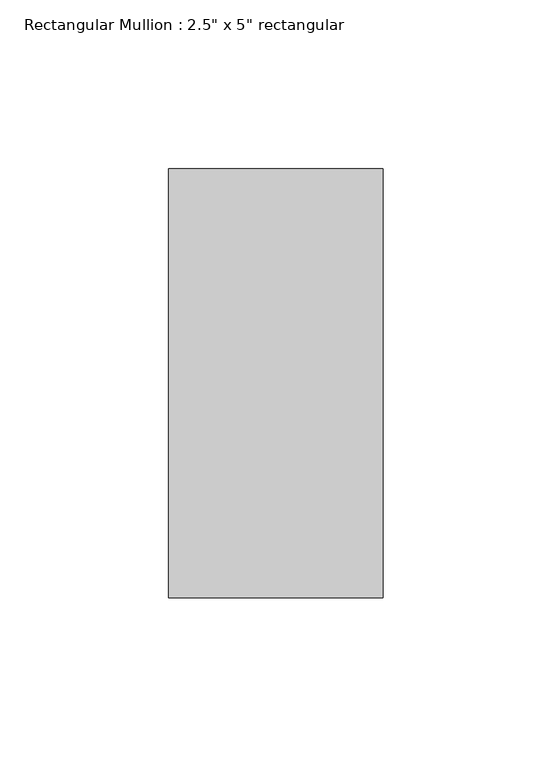
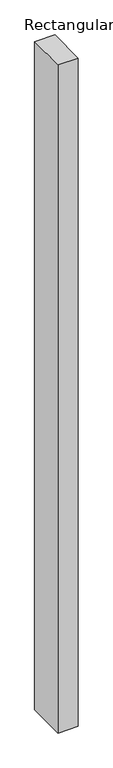
"""IFC4 building model written with IfcOpenShell, lengths in millimetres: member geometry."""

from ifc_helpers import new_model, si_unit, frame, origin, place, context, project, spatial, polyline, outline, extrude, source, transform, mapped, element, save


def member_4e4be739(model_context):
    return source(origin(), model_context, "Body", "SweptSolid", [
        extrude(outline(polyline([(0.0, 63.5), (0.0, -63.5), (-63.5, -63.5), (-63.5, 63.5), (0.0, 63.5)])), frame((0.0, 0.0, -2220.4042846), z_axis=(0.0, 0.0, 1.0), x_axis=(1.0, 0.0, 0.0)), (0.0, 0.0, 1.0), 2220.4042846),
    ])


if __name__ == "__main__":
    model = new_model("IFC4")
    model_context = context("Model", 3, world=origin())
    ifc_project = project(units=[si_unit("LENGTHUNIT", "METRE", prefix="MILLI")], contexts=[model_context])
    site = spatial("IfcSite", under=ifc_project)
    building = spatial("IfcBuilding", under=site)
    placement = place(None, origin())
    member_shape = member_4e4be739(model_context)
    element("IfcMember", 1, ObjectType="Rectangular Mullion : 2.5\" x 5\" rectangular", at=placement, inside=building, context=model_context, shape_type="MappedRepresentation", body=[
        mapped(member_shape, transform((0.0, 0.0, 0.0), x_axis=(1.0, 0.0, 0.0), y_axis=(0.0, 1.0, 0.0), z_axis=(0.0, 0.0, 1.0))),
    ])
    save(model, "model.ifc")

# Revit data of these elements
# Type "Rectangular Mullion : 2.5\" x 5\" rectangular"
#   built-in parameter 1007304 = 0.416667 (stored number, unit not read)
#   built-in parameter 1007301 = 0.104167 (stored number, unit not read)
#   built-in parameter 1007300 = 0.104167 (stored number, unit not read)
